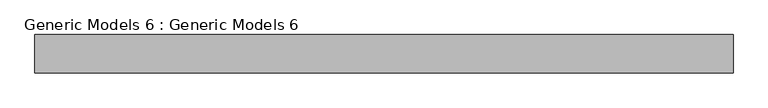
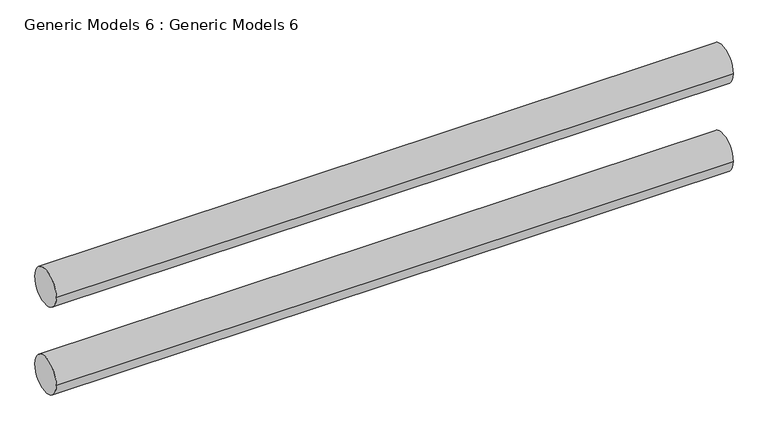
"""IFC4 building model written with IfcOpenShell, lengths in millimetres: proxy geometry, Generic Models 6 : Generic Models 6."""

from ifc_helpers import new_model, si_unit, point, frame, frame_2d, origin, place, context, project, spatial, circle_curve, trimmed, segment, composite_curve, outline, extrude, source, transform, mapped, element, save


def generic_models_6_generic_models_6_15436f46(model_context):
    return source(origin(), model_context, "Body", "SweptSolid", [
        extrude(outline(composite_curve([segment(trimmed(circle_curve(frame_2d((-8631.4820248, 10662.9725082)), 127.0), [point((-8758.4820248, 10662.9725082))], [point((-8504.4820248, 10662.9725082))], False, "CARTESIAN"), True, "CONTINUOUS"), segment(trimmed(circle_curve(frame_2d((-8631.4820248, 10662.9725082)), 127.0), [point((-8504.4820248, 10662.9725082))], [point((-8758.4820248, 10662.9725082))], False, "CARTESIAN"), True, "CONTINUOUS")], self_intersect=False)), frame((619.665012, 0.0, 0.0), z_axis=(1.0, 0.0, 0.0), x_axis=(0.0, 1.0, 0.0)), (0.0, 0.0, 1.0), 4627.4934796),
        extrude(outline(composite_curve([segment(trimmed(circle_curve(frame_2d((-8631.4820248, 10027.9725082)), 127.0), [point((-8758.4820248, 10027.9725082))], [point((-8504.4820248, 10027.9725082))], False, "CARTESIAN"), True, "CONTINUOUS"), segment(trimmed(circle_curve(frame_2d((-8631.4820248, 10027.9725082)), 127.0), [point((-8504.4820248, 10027.9725082))], [point((-8758.4820248, 10027.9725082))], False, "CARTESIAN"), True, "CONTINUOUS")], self_intersect=False)), frame((619.665012, 0.0, 0.0), z_axis=(1.0, 0.0, 0.0), x_axis=(0.0, 1.0, 0.0)), (0.0, 0.0, 1.0), 4627.4934796),
    ])


if __name__ == "__main__":
    model = new_model("IFC4")
    model_context = context("Model", 3, world=origin())
    ifc_project = project(units=[si_unit("LENGTHUNIT", "METRE", prefix="MILLI")], contexts=[model_context])
    site = spatial("IfcSite", under=ifc_project)
    building = spatial("IfcBuilding", under=site)
    placement = place(None, origin())
    generic_models_6_generic_models_6_shape = generic_models_6_generic_models_6_15436f46(model_context)
    element("IfcBuildingElementProxy", 1, Name="Generic Models 6 : Generic Models 6", ObjectType="Generic Models 6 : Generic Models 6", at=placement, inside=building, context=model_context, shape_type="MappedRepresentation", body=[
        mapped(generic_models_6_generic_models_6_shape, transform((0.0, 0.0, 0.0), x_axis=(1.0, 0.0, 0.0), y_axis=(0.0, 1.0, 0.0), z_axis=(0.0, 0.0, 1.0))),
    ])
    save(model, "model.ifc")

# Revit data of these elements
# Element 1 (IfcBuildingElementProxy, "Generic Models 6 : Generic Models 6")
#   Materials on its faces: "Brick, Soldier Course"
# Materials
#   "Brick, Soldier Course": class "Masonry", colour RGB 170 98 104, transparency 0, Description = "Common brick soldier coursed", Cost = 0
